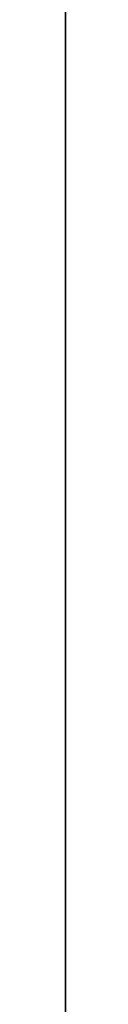
# Model space of a CAD drawing. Units: inches. Extents: x 2083 to 3317, y 1141 to 2115.
# Tile 31 of 256: x 2235.95969 to 2235.95984, y 1477.76912 to 1477.77958. Entities that reach past the tile are written whole.
import ezdxf

# ---------------------------------------------------------------- set-up
doc = ezdxf.new("R2010")
doc.units = ezdxf.units.IN
doc.layers.add('A-ANNO-DIMS', color=2, linetype='Continuous', lineweight=18)
doc.layers.add('A-WALL', color=7, linetype='Continuous', lineweight=35)
doc.layers.add('A-WALL-PATT', color=251, linetype='Continuous', lineweight=13, true_color=0x636466)
doc.styles.get("Standard").update_dxf_attribs({"font": 'arial.ttf'})
doc.dimstyles.new('ISO-25', dxfattribs={"dimtxt": 12, "dimasz": 12, "dimexe": 1.25, "dimexo": 0.625, "dimtad": 1, "dimlunit": 3, "dimtxsty": 'Standard', "dimcen": 2.5, "dimadec": 0, "dimazin": 0, "dimtfac": 1, "dimtmove": 0, "dimatfit": 3, "dimfxl": 1, "dimarcsym": 0})

# ---------------------------------------------------------------- blocks, each defined once
blk = doc.blocks.new('*D30')
at = {"layer": 'A-ANNO-DIMS', "color": 0, "lineweight": -2, "transparency": 16777216}
for p, q in [((2240.017856, 1445.273807), (2240.017856, 1448.045528)), ((2254.329327, 1445.273807), (2254.329327, 1448.045528)), ((2228.017856, 1446.795528), (2216.017856, 1446.795528)), ((2240.017856, 1446.795528), (2254.329327, 1446.795528)), ((2266.329327, 1446.795528), (2413.764866, 1446.795528))]:
    blk.add_line(p, q, dxfattribs=at)
at = {"layer": 'A-ANNO-DIMS', "color": 0, "transparency": 16777216}
for points in [[(2228.017856, 1448.795528), (2228.017856, 1444.795528), (2240.017856, 1446.795528)], [(2266.329327, 1448.795528), (2266.329327, 1444.795528), (2254.329327, 1446.795528)]]:
    blk.add_solid(points, dxfattribs=at)
at = {"layer": 'Defpoints', "color": 0, "transparency": 16777216}
for p in [(2254.329327, 1446.795528), (2240.017856, 1444.648807), (2254.329327, 1444.648807)]:
    blk.add_point(p, dxfattribs=at)
at = {"layer": 'A-ANNO-DIMS', "color": 0, "transparency": 16777216, "insert": (2346.047096, 1453.625167), "char_height": 12, "attachment_point": 5}
blk.add_mtext('WC 1\'-2 1/2" TYP.', dxfattribs=at)
blk = doc.blocks.new('*D31')
at = {"layer": 'A-ANNO-DIMS', "color": 0, "lineweight": -2, "transparency": 16777216}
for p, q in [((2237.871136, 1456.648807), (2237.871136, 1541.915179)), ((2239.392856, 1444.648807), (2236.621136, 1444.648807)), ((2237.871136, 1431.547542), (2237.871136, 1444.648807)), ((2239.392856, 1431.547542), (2236.621136, 1431.547542)), ((2237.871136, 1419.547542), (2237.871136, 1407.547542))]:
    blk.add_line(p, q, dxfattribs=at)
at = {"layer": 'A-ANNO-DIMS', "color": 0, "transparency": 16777216}
for points in [[(2235.871136, 1456.648807), (2239.871136, 1456.648807), (2237.871136, 1444.648807)], [(2235.871136, 1419.547542), (2239.871136, 1419.547542), (2237.871136, 1431.547542)]]:
    blk.add_solid(points, dxfattribs=at)
at = {"layer": 'Defpoints', "color": 0, "transparency": 16777216}
for p in [(2237.871136, 1444.648807), (2240.017856, 1444.648807), (2240.017856, 1431.547542)]:
    blk.add_point(p, dxfattribs=at)
at = {"layer": 'A-ANNO-DIMS', "color": 0, "transparency": 16777216, "insert": (2231.217486, 1505.281993), "char_height": 12, "attachment_point": 5, "rotation": 90}
blk.add_mtext('1\'-1" TYP.', dxfattribs=at)
blk = doc.blocks.new('*D45')
at = {"layer": 'A-ANNO-DIMS', "color": 0, "lineweight": -2, "transparency": 16777216}
for p, q in [((2235.959783, 1478.38636), (2235.959783, 1531.36136)), ((2418.959783, 1478.38636), (2418.959783, 1531.36136)), ((2247.959783, 1530.11136), (2406.959783, 1530.11136))]:
    blk.add_line(p, q, dxfattribs=at)
at = {"layer": 'A-ANNO-DIMS', "color": 0, "transparency": 16777216}
for points in [[(2247.959783, 1532.11136), (2247.959783, 1528.11136), (2235.959783, 1530.11136)], [(2406.959783, 1532.11136), (2406.959783, 1528.11136), (2418.959783, 1530.11136)]]:
    blk.add_solid(points, dxfattribs=at)
at = {"layer": 'Defpoints', "color": 0, "transparency": 16777216}
for p in [(2418.959783, 1530.11136), (2235.959783, 1477.76136), (2418.959783, 1477.76136)]:
    blk.add_point(p, dxfattribs=at)
at = {"layer": 'A-ANNO-DIMS', "color": 0, "transparency": 16777216, "insert": (2327.459783, 1536.867329), "char_height": 12, "attachment_point": 5}
blk.add_mtext('15\'-3"', dxfattribs=at)
blk = doc.blocks.new('*D62')
at = {"layer": 'A-ANNO-DIMS', "color": 0, "lineweight": -2, "transparency": 16777216}
for p, q in [((2235.959783, 1469.38636), (2235.959783, 1522.36136)), ((2379.959783, 1469.38636), (2379.959783, 1522.36136)), ((2247.959783, 1521.11136), (2367.959783, 1521.11136))]:
    blk.add_line(p, q, dxfattribs=at)
at = {"layer": 'A-ANNO-DIMS', "color": 0, "transparency": 16777216}
for points in [[(2247.959783, 1523.11136), (2247.959783, 1519.11136), (2235.959783, 1521.11136)], [(2367.959783, 1523.11136), (2367.959783, 1519.11136), (2379.959783, 1521.11136)]]:
    blk.add_solid(points, dxfattribs=at)
at = {"layer": 'Defpoints', "color": 0, "transparency": 16777216}
for p in [(2379.959783, 1521.11136), (2235.959783, 1468.76136), (2379.959783, 1468.76136)]:
    blk.add_point(p, dxfattribs=at)
at = {"layer": 'A-ANNO-DIMS', "color": 0, "transparency": 16777216, "insert": (2307.959783, 1527.863236), "char_height": 12, "attachment_point": 5}
blk.add_mtext('12\'-0"', dxfattribs=at)

msp = doc.modelspace()

# ---------------------------------------------------------------- hatches: boundary and pattern name
at = {"layer": 'A-WALL-PATT'}
h = msp.add_hatch(color=256, dxfattribs=at)
h.dxf.hatch_style = 1
h.paths.add_polyline_path([(3126.959783, 2020.76136), (2748.959783, 2020.76136), (2604.959783, 2020.76136), (2226.959783, 2020.76136), (2226.959783, 1702.76136), (2466.959783, 1702.76136), (2466.959783, 1582.76136), (2418.959783, 1582.76136), (2418.959783, 1477.76136), (2226.959783, 1477.76136), (2226.959783, 1263.26136), (2544.959783, 1263.26136), (2544.959783, 1411.76136), (2604.959783, 1411.76136), (2685.959783, 1411.76136), (2685.959783, 1420.76136), (2604.959783, 1420.76136), (2604.959783, 1573.76136), (2604.959783, 1702.76136), (2604.959783, 2011.76136), (2748.959783, 2011.76136), (2748.959783, 1702.76136), (2862.959783, 1702.76136), (2862.959783, 1621.76136), (2871.959783, 1621.76136), (2871.959783, 1702.76136), (2883.959783, 1702.76136), (2883.959783, 1706.939459, -0.026459), (2883.959783, 1711.76136), (2757.959783, 1711.76136), (2757.959783, 1807.76136), (2787.959783, 1807.76136), (2787.959783, 1812.26136), (2757.959783, 1812.26136), (2757.959783, 2011.76136), (2877.959783, 2011.76136), (2877.959783, 1812.26136), (2847.959783, 1812.26136), (2847.959783, 1807.76136), (2889.835742, 1807.76136), (2889.835742, 1812.26136), (2882.459783, 1812.26136), (2882.459783, 2011.76136), (3117.959783, 2011.76136), (3117.959783, 1812.26136), (2937.835742, 1812.26136), (2937.835742, 1807.76136), (2995.709783, 1807.76136), (2995.709783, 1796.117666), (3000.209783, 1796.117666), (3000.209783, 1807.76136), (3117.959783, 1807.76136), (3117.959783, 1711.76136), (3000.209783, 1711.76136), (3000.209783, 1760.117666), (2998.572705, 1760.117666, -0.020711), (2995.709783, 1760.117666), (2995.709783, 1711.76136), (2931.959783, 1711.76136), (2931.959783, 1702.76136), (3126.959783, 1702.76136)])
h.paths.add_polyline_path([(2471.459783, 2011.76136), (2471.459783, 1810.01136), (2462.716936, 1810.01136), (2462.716936, 1805.51136), (2505.959783, 1805.51136), (2505.959783, 1810.01136), (2475.959783, 1810.01136), (2475.959783, 2011.76136), (2595.959783, 2011.76136), (2595.959783, 1810.01136), (2565.959783, 1810.01136), (2565.959783, 1805.51136), (2595.959783, 1805.51136), (2595.959783, 1711.76136), (2235.959783, 1711.76136), (2235.959783, 1805.51136), (2353.709783, 1805.51136), (2353.709783, 1796.054162), (2358.209783, 1796.054162), (2358.209783, 1805.51136), (2414.716936, 1805.51136), (2414.716936, 1810.01136), (2235.959783, 1810.01136), (2235.959783, 2011.76136)], flags=16)
h.paths.add_polyline_path([(2270.204734, 1994.610008), (2270.204734, 1970.610008), (2246.204734, 1970.610008), (2246.204734, 1994.610008)], flags=0)
edge = h.paths.add_edge_path(flags=0)
edge.add_ellipse((2332.027391, 1899.798176), major_axis=(-3.042994, 3.042994), ratio=0.16825245, start_angle=-161.332166, end_angle=-156.307114, ccw=False)
edge.add_ellipse((2333.082037, 1898.74353), major_axis=(-1.054646, 1.054646), ratio=0.4535321, start_angle=-123.371019, end_angle=-94.159107)
edge = h.paths.add_edge_path(flags=0)
edge.add_ellipse((2332.027391, 1968.87629), major_axis=(3.042994, 3.042994), ratio=0.16825245, start_angle=18.667834, end_angle=23.692886)
edge.add_spline(control_points=[(2332.925596, 1970.691105), (2332.226768, 1970.3361), (2330.893709, 1969.658905), (2328.41308, 1970.932138), (2327.203934, 1967.748712), (2324.709596, 1969.955589), (2322.532822, 1967.012354), (2320.012846, 1971.295812), (2317.680308, 1968.157845), (2316.040526, 1967.102047), (2315.426904, 1966.809602)], knot_values=[0, 0, 0, 0, 2.267059, 4.324559, 6.685584, 8.878641, 11.121502, 14.300359, 17.755284, 19.732645, 19.732645, 19.732645, 19.732645], degree=3, periodic=0)
edge.add_ellipse((2332.027391, 1968.87629), major_axis=(3.042994, 3.042994), ratio=0.16825245, start_angle=18.667834, end_angle=23.692886, ccw=False)
edge.add_ellipse((2333.082037, 1969.930936), major_axis=(1.054646, 1.054646), ratio=0.4535321, start_angle=56.628981, end_angle=85.840893, ccw=False)
edge = h.paths.add_edge_path(flags=0)
edge.add_spline(control_points=[(2296.428287, 1967.987908), (2293.627804, 1965.336314), (2287.703624, 1959.727094), (2299.74386, 1949.995699), (2294.532591, 1935.668528), (2290.573228, 1920.603512), (2293.394124, 1909.973691), (2296.185407, 1904.966543)], knot_values=[0.099185, 0.099185, 0.099185, 0.099185, 0.345301, 0.619822, 0.982653, 1.386093, 1.810555, 1.810555, 1.810555, 1.810555], degree=3, periodic=0)
edge.add_spline(control_points=[(2296.185407, 1904.966543), (2297.383582, 1902.6193), (2298.000969, 1901.949312), (2298.55297, 1901.468155)], knot_values=[0.006246, 0.006246, 0.006246, 0.006246, 0.055476, 0.055476, 0.055476, 0.055476], degree=3, periodic=0)
edge.add_spline(control_points=[(2298.55297, 1901.468155), (2297.258612, 1900.923224), (2295.225294, 1900.232126), (2293.060229, 1900.614205), (2292.101423, 1900.788415), (2292.089578, 1900.790568)], knot_values=[0.312835, 0.312835, 0.312835, 0.312835, 0.40178, 0.474987, 0.475903, 0.475903, 0.475903, 0.475903], degree=3, periodic=0)
edge.add_arc((2292.793646, 1904.664109), 3.937008, 215.420897, 259.698179, ccw=False)
edge.add_spline(control_points=[(2289.585314, 1902.382304), (2289.476652, 1902.535087), (2289.36848, 1902.688035), (2289.260865, 1902.84117)], knot_values=[0.102872, 0.102872, 0.102872, 0.102872, 0.116896, 0.116896, 0.116896, 0.116896], degree=3, periodic=0)
edge.add_spline(control_points=[(2289.260865, 1902.84117), (2288.686604, 1902.550192), (2287.640048, 1902.019902), (2285.881337, 1901.873954), (2283.852972, 1901.504352), (2281.719987, 1899.710538), (2278.466991, 1899.492942), (2276.157136, 1901.883202), (2272.258953, 1899.804071), (2267.777605, 1901.843183), (2262.243882, 1900.184033), (2257.414927, 1901.782061), (2254.318374, 1900.72612), (2253.178285, 1900.337343)], knot_values=[0, 0, 0, 0, 1.907977, 3.477176, 5.261074, 7.972851, 11.680248, 13.717921, 16.939592, 22.789562, 27.502503, 33.595215, 37.145618, 37.145618, 37.145618, 37.145618], degree=3, periodic=0)
edge.add_line((2253.178285, 1900.337343), (2250.24424, 1902.84117))
edge.add_line((2250.24424, 1902.84117), (2250.24424, 1965.833296))
edge.add_line((2250.24424, 1965.833296), (2253.178285, 1968.337123))
edge.add_spline(control_points=[(2253.178285, 1968.337123), (2254.318374, 1967.948346), (2257.414927, 1966.892405), (2262.243882, 1968.490433), (2267.777605, 1966.831283), (2271.52673, 1968.537217), (2273.875914, 1967.828289), (2274.206701, 1967.727642)], knot_values=[0, 0, 0, 0, 0.09018, 0.244935, 0.364644, 0.513233, 0.537855, 0.537855, 0.537855, 0.537855], degree=3, periodic=0)
edge.add_arc((2274.352887, 1963.793349), 3.937008, 72.051134, 92.127949, ccw=False)
edge.add_arc((2281.296933, 1985.230003), 18.596298, 252.0511336, 288.5657217)
edge.add_arc((2292.316717, 1956.02888), 12.646081, 71.0267879, 113.7782184, ccw=False)
edge = h.paths.add_edge_path(flags=0)
edge.add_spline(control_points=[(2274.899415, 1951.856195), (2275.066156, 1951.616592), (2275.232687, 1951.376588), (2275.397987, 1951.135855)], knot_values=[1.409916, 1.409916, 1.409916, 1.409916, 1.43159, 1.43159, 1.43159, 1.43159], degree=3, periodic=0)
edge.add_spline(control_points=[(2275.397987, 1951.135855), (2275.792106, 1950.561885), (2276.179231, 1949.983774), (2276.545546, 1949.397103)], knot_values=[1.358238, 1.358238, 1.358238, 1.358238, 1.409916, 1.409916, 1.409916, 1.409916], degree=3, periodic=0)
edge.add_line((2276.545546, 1949.397103), (2277.437289, 1947.862185))
edge.add_spline(control_points=[(2277.437289, 1947.862185), (2276.303834, 1945.673115), (2274.639698, 1942.426882), (2274.631615, 1938.0939), (2272.799124, 1930.85155), (2274.356426, 1943.897046), (2275.947681, 1947.923356), (2276.545546, 1949.397103)], knot_values=[0.005632, 0.005632, 0.005632, 0.005632, 0.186014, 0.266002, 0.357087, 0.59639, 0.739732, 0.739732, 0.739732, 0.739732], degree=3, periodic=0)
edge.add_spline(control_points=[(2276.545546, 1949.397103), (2276.179231, 1949.983774), (2275.792106, 1950.561885), (2275.397987, 1951.135855)], knot_values=[1.358238, 1.358238, 1.358238, 1.358238, 1.409916, 1.409916, 1.409916, 1.409916], degree=3, periodic=0)
edge.add_spline(control_points=[(2275.397987, 1951.135855), (2274.9425, 1950.080452), (2274.20776, 1948.025272), (2273.934602, 1944.851477), (2272.468534, 1937.627489), (2273.466216, 1945.696466), (2274.700615, 1951.059472), (2274.899415, 1951.856195)], knot_values=[0.104364, 0.104364, 0.104364, 0.104364, 0.189636, 0.269624, 0.36071, 0.600013, 0.644622, 0.644622, 0.644622, 0.644622], degree=3, periodic=0)
h.paths.add_polyline_path([(2269.167514, 1963.127573, -0.357527), (2268.170633, 1960.97637, -0.092561), (2268.170633, 1939.436325, -0.357527), (2269.167514, 1937.285122, -0.357527), (2267.01631, 1938.282002, -0.164785), (2254.685581, 1938.282002, -0.357527), (2252.534378, 1937.285122, -0.357527), (2253.531259, 1939.436325, -0.092561), (2253.531259, 1960.97637, -0.357527), (2252.534378, 1963.127573, -0.357527), (2254.685581, 1962.130692, -0.164785), (2267.01631, 1962.130692, -0.357527)], flags=0)
h.paths.add_polyline_path([(2248.874068, 1967.8018), (2248.874068, 1957.02771), (2249.457783, 1957.02771), (2249.457783, 1911.646756), (2248.874068, 1911.646756), (2248.874068, 1900.872666), (2246.511863, 1900.872666, 0.197327), (2244.149658, 1902.456873), (2244.149658, 1966.217592, 0.197327), (2246.511863, 1967.8018)], flags=0)
h.paths.add_polyline_path([(2269.167514, 1931.389344, -0.357527), (2268.170633, 1929.238141, -0.092561), (2268.170633, 1907.698096, -0.357527), (2269.167514, 1905.546893, -0.357527), (2267.01631, 1906.543774, -0.164785), (2254.685581, 1906.543774, -0.357527), (2252.534378, 1905.546893, -0.357527), (2253.531259, 1907.698096, -0.092561), (2253.531259, 1929.238141, -0.357527), (2252.534378, 1931.389344, -0.357527), (2254.685581, 1930.392463, -0.164785), (2267.01631, 1930.392463, -0.357527)], flags=0)
edge = h.paths.add_edge_path(flags=0)
edge.add_spline(control_points=[(2276.196858, 1906.723702), (2276.168144, 1909.028928), (2276.114049, 1913.371852), (2270.598417, 1924.924978), (2273.905175, 1919.012779), (2275.921711, 1916.262063), (2275.47457, 1912.402149), (2277.257874, 1910.380621), (2276.696044, 1908.225036), (2276.646218, 1906.813023), (2276.617825, 1906.008407)], knot_values=[0, 0, 0, 0, 8.61026, 16.221274, 18.843057, 23.804898, 27.440828, 29.356102, 31.203478, 33.650687, 33.650687, 33.650687, 33.650687], degree=3, periodic=0)
edge.add_spline(control_points=[(2276.617825, 1906.008407), (2276.623313, 1905.624144), (2276.497738, 1904.628661), (2275.441779, 1903.854725), (2274.937314, 1903.08045), (2274.85908, 1902.84117)], knot_values=[0.156488, 0.156488, 0.156488, 0.156488, 0.184398, 0.231376, 0.250598, 0.250598, 0.250598, 0.250598], degree=3, periodic=0)
edge.add_line((2274.85908, 1902.84117), (2276.50598, 1902.84117))
edge.add_spline(control_points=[(2276.50598, 1902.84117), (2276.788308, 1903.08494), (2277.665071, 1904.125196), (2278.249538, 1904.340738), (2277.653872, 1908.527387), (2278.15567, 1906.227808), (2278.100464, 1905.285948), (2278.846675, 1904.069005), (2277.856785, 1903.414948), (2277.874191, 1902.99105), (2277.903562, 1902.84117)], knot_values=[0.059574, 0.059574, 0.059574, 0.059574, 0.080753, 0.103741, 0.16972, 0.176036, 0.207137, 0.240474, 0.262341, 0.27366, 0.27366, 0.27366, 0.27366], degree=3, periodic=0)
edge.add_line((2277.903562, 1902.84117), (2280.029825, 1902.84117))
edge.add_spline(control_points=[(2280.029825, 1902.84117), (2279.888221, 1903.088398), (2279.499257, 1903.981551), (2280.152284, 1905.939349), (2278.103615, 1909.657757), (2279.762395, 1907.185285), (2280.3279, 1904.874861), (2280.485109, 1903.48959), (2281.463269, 1903.249432), (2281.758343, 1902.936497), (2281.834036, 1902.84117)], knot_values=[0.013856, 0.013856, 0.013856, 0.013856, 0.034874, 0.088867, 0.107879, 0.126738, 0.158714, 0.193757, 0.217487, 0.226722, 0.226722, 0.226722, 0.226722], degree=3, periodic=0)
edge.add_spline(control_points=[(2281.834036, 1902.84117), (2281.787535, 1902.826703), (2281.647022, 1902.782988), (2281.395527, 1902.85949), (2281.088077, 1902.985242), (2280.720683, 1903.060902), (2280.333451, 1903.025726), (2280.124767, 1902.898879), (2280.029825, 1902.84117)], knot_values=[0, 0, 0, 0, 0.14413, 0.435517, 0.749276, 1.153046, 1.548371, 1.878348, 1.878348, 1.878348, 1.878348], degree=3, periodic=0)
edge.add_line((2280.029825, 1902.84117), (2277.903562, 1902.84117))
edge.add_spline(control_points=[(2277.903562, 1902.84117), (2277.892855, 1902.795855), (2277.865396, 1902.679637), (2277.607479, 1902.687483), (2277.27405, 1902.8007), (2276.837921, 1902.619775), (2276.583807, 1902.789261), (2276.50598, 1902.84117)], knot_values=[0, 0, 0, 0, 0.127189, 0.326199, 0.628009, 1.24357, 1.515331, 1.515331, 1.515331, 1.515331], degree=3, periodic=0)
edge.add_line((2276.50598, 1902.84117), (2274.85908, 1902.84117))
edge.add_spline(control_points=[(2274.85908, 1902.84117), (2274.814437, 1902.898587), (2274.72513, 1903.013446), (2274.493477, 1903.118968), (2274.244285, 1902.960539), (2273.937121, 1903.184942), (2273.614039, 1902.983143), (2273.408316, 1902.883045), (2273.322254, 1902.84117)], knot_values=[0, 0, 0, 0, 0.21843, 0.436957, 0.687977, 0.990379, 1.398396, 1.69185, 1.69185, 1.69185, 1.69185], degree=3, periodic=0)
edge.add_spline(control_points=[(2273.322254, 1902.84117), (2273.61674, 1903.445692), (2274.273998, 1904.538253), (2276.027239, 1904.573702), (2276.206963, 1906.583637), (2276.196858, 1906.723702)], knot_values=[0.012227, 0.012227, 0.012227, 0.012227, 0.059472, 0.106218, 0.134458, 0.134458, 0.134458, 0.134458], degree=3, periodic=0)
h.paths.add_polyline_path([(2270.776054, 1897.789828), (2270.776054, 1873.789828), (2246.776054, 1873.789828), (2246.776054, 1897.789828)], flags=0)
h.paths.add_polyline_path([(2353.709783, 1760.005059), (2353.709783, 1760.054162), (2358.209783, 1760.054162, -0.033729)], flags=0)
h.paths.add_polyline_path([(2321.819119, 1737.529186), (2341.995327, 1737.529186, -0.414214), (2343.203273, 1736.321241), (2343.203273, 1721.020596, -0.414214), (2341.995327, 1719.812651), (2321.819119, 1719.812651, -0.414214), (2320.611173, 1721.020596), (2320.611173, 1736.321241, -0.414214)], flags=0)
h.paths.add_polyline_path([(2324.23501, 1736.321241), (2339.579436, 1736.321241, -0.414214), (2341.995327, 1733.905349), (2341.995327, 1725.44973, -0.414214), (2339.579436, 1723.033839), (2333.680588, 1723.033839), (2333.845317, 1722.045467, -0.870646), (2335.425399, 1721.825893, -0.767327), (2333.922694, 1721.423245), (2331.291024, 1721.423245, -0.767327), (2329.788319, 1721.825893, -0.870646), (2331.368401, 1722.045467), (2331.53313, 1723.033839), (2324.23501, 1723.033839, -0.414214), (2321.819119, 1725.44973), (2321.819119, 1733.905349, -0.414214)], flags=0)
h.paths.add_polyline_path([(2570.483789, 1928.615444), (2589.683789, 1928.615444), (2590.168829, 1928.615444), (2590.168829, 1904.993397), (2570.483789, 1904.993397)], flags=0)
h.paths.add_polyline_path([(2574.447324, 1927.263822, -1), (2572.828836, 1927.263822, -1)], flags=0)
h.paths.add_polyline_path([(2573.089867, 1926.940877), (2573.925032, 1927.776042), (2574.147743, 1927.553332), (2573.312577, 1926.718166)], flags=0)
h.paths.add_polyline_path([(2578.779065, 1919.729618, -1), (2571.591663, 1919.729618, -1)], flags=0)
h.paths.add_polyline_path([(2578.385364, 1919.729618, -1), (2571.985364, 1919.729618, -1)], flags=0)
h.paths.add_polyline_path([(2331.595764, 1729.476216, -1), (2333.617954, 1729.476216, -1)], flags=0)
h.paths.add_polyline_path([(2578.034228, 1927.263822, -1), (2576.41574, 1927.263822, -1)], flags=0)
h.paths.add_polyline_path([(2576.688851, 1927.531089), (2576.911562, 1927.753799), (2577.746728, 1926.918634), (2577.524017, 1926.695923)], flags=0)
h.paths.add_polyline_path([(2578.139065, 1909.859539, -1), (2572.231663, 1909.859539, -1)], flags=0)
h.paths.add_polyline_path([(2577.745364, 1909.859539, -1), (2572.625364, 1909.859539, -1)], flags=0)
h.paths.add_polyline_path([(2583.797718, 1927.263822, -1), (2582.179229, 1927.263822, -1)], flags=0)
h.paths.add_polyline_path([(2582.718649, 1927.753799), (2583.553814, 1926.918634), (2583.331103, 1926.695923), (2582.495938, 1927.531089)], flags=0)
h.paths.add_polyline_path([(2582.495938, 1927.531089), (2582.718649, 1927.753799), (2583.553814, 1926.918634), (2583.331103, 1926.695923)], flags=0)
h.paths.add_polyline_path([(2587.739065, 1920.529618, -1), (2581.831663, 1920.529618, -1)], flags=0)
h.paths.add_polyline_path([(2587.345364, 1920.529618, -1), (2582.225364, 1920.529618, -1)], flags=0)
h.paths.add_polyline_path([(2587.384622, 1927.263822, -1), (2585.766133, 1927.263822, -1)], flags=0)
h.paths.add_polyline_path([(2586.081993, 1926.980247), (2586.917158, 1927.815412), (2587.139869, 1927.592702), (2586.304703, 1926.757536)], flags=0)
h.paths.add_polyline_path([(2588.379065, 1910.659539, -1), (2581.191663, 1910.659539, -1)], flags=0)
h.paths.add_polyline_path([(2587.985364, 1910.659539, -1), (2581.585364, 1910.659539, -1)], flags=0)
h.paths.add_polyline_path([(2417.167729, 1729.477895), (2437.343937, 1729.477895, -0.414214), (2438.551883, 1728.26995), (2438.551883, 1712.969306, -0.414214), (2437.343937, 1711.76136), (2417.167729, 1711.76136, -0.414214), (2415.959783, 1712.969306), (2415.959783, 1728.26995, -0.414214)], flags=0)
h.paths.add_polyline_path([(2419.58362, 1728.26995), (2434.928046, 1728.26995, -0.414214), (2437.343937, 1725.854059), (2437.343937, 1717.39844, -0.414214), (2434.928046, 1714.982548), (2429.029199, 1714.982548), (2429.193927, 1713.994176, -0.870646), (2430.774009, 1713.774603, -0.767327), (2429.271304, 1713.371954), (2426.639634, 1713.371954, -0.767327), (2425.136929, 1713.774603, -0.870646), (2426.717011, 1713.994176), (2426.88174, 1714.982548), (2419.58362, 1714.982548, -0.414214), (2417.167729, 1717.39844), (2417.167729, 1725.854059, -0.414214)], flags=0)
h.paths.add_polyline_path([(2419.58362, 1728.26995), (2434.928046, 1728.26995, -0.414214), (2437.343937, 1725.854059), (2437.343937, 1717.39844, -0.414214), (2434.928046, 1714.982548), (2429.029199, 1714.982548), (2428.358118, 1719.009034), (2427.552821, 1719.009034), (2426.88174, 1714.982548), (2419.58362, 1714.982548, -0.414214), (2417.167729, 1717.39844), (2417.167729, 1725.854059, -0.414214)], flags=0)
h.paths.add_polyline_path([(2426.944374, 1721.424925, -1), (2428.966564, 1721.424925, -1)], flags=0)
h.paths.add_polyline_path([(2475.959783, 1702.76136), (2595.959783, 1702.76136), (2595.959783, 1582.76136), (2475.959783, 1582.76136)], flags=16)
h.paths.add_polyline_path([(2427.959783, 1573.76136), (2595.959783, 1573.76136), (2595.959783, 1468.76136), (2595.959783, 1420.76136), (2384.459783, 1420.76136), (2384.459783, 1468.76136), (2427.959783, 1468.76136)], flags=16)
h.paths.add_polyline_path([(2379.959783, 1468.76136), (2379.959783, 1420.76136), (2235.959783, 1420.76136), (2235.959783, 1468.76136)], flags=16)
h.paths.add_polyline_path([(2317.815996, 1466.695767), (2337.992205, 1466.695767, -0.414214), (2339.20015, 1465.487821), (2339.20015, 1450.187177, -0.414214), (2337.992205, 1448.979232), (2317.815996, 1448.979232, -0.414214), (2316.608051, 1450.187177), (2316.608051, 1465.487821, -0.414214)], flags=0)
h.paths.add_polyline_path([(2320.231887, 1465.487821), (2335.576313, 1465.487821, -0.414214), (2337.992205, 1463.07193), (2337.992205, 1454.616311, -0.414214), (2335.576313, 1452.20042), (2329.677466, 1452.20042), (2329.842195, 1451.212047, -0.870646), (2331.422276, 1450.992474, -0.767327), (2329.919571, 1450.589826), (2327.287902, 1450.589826, -0.767327), (2325.785197, 1450.992474, -0.870646), (2327.365278, 1451.212047), (2327.530007, 1452.20042), (2320.231887, 1452.20042, -0.414214), (2317.815996, 1454.616311), (2317.815996, 1463.07193, -0.414214)], flags=0)
h.paths.add_polyline_path([(2320.231887, 1465.487821), (2335.576313, 1465.487821, -0.414214), (2337.992205, 1463.07193), (2337.992205, 1454.616311, -0.414214), (2335.576313, 1452.20042), (2329.677466, 1452.20042), (2329.006385, 1456.226905), (2328.201088, 1456.226905), (2327.530007, 1452.20042), (2320.231887, 1452.20042, -0.414214), (2317.815996, 1454.616311), (2317.815996, 1463.07193, -0.414214)], flags=0)
h.paths.add_polyline_path([(2327.592641, 1458.642796, -1), (2329.614832, 1458.642796, -1)], flags=0)
h.paths.add_polyline_path([(2244.411744, 1433.340453), (2241.920945, 1433.340453, -0.414214), (2240.017856, 1435.243542), (2240.017856, 1440.952808, -0.414211), (2241.920925, 1442.855897), (2244.411744, 1442.855897, -1.976472)], flags=0)
h.paths.add_polyline_path([(2245.356888, 1434.397536, -0.414214), (2245.356888, 1441.798814, -2.144098)], flags=0)
h.paths.add_polyline_path([(2535.959783, 1416.26136), (2535.959783, 1272.26136), (2235.959783, 1272.26136), (2235.959783, 1416.26136)], flags=16)
h.paths.add_polyline_path([(2260.119561, 1384.292841), (2260.119561, 1362.038649), (2237.865369, 1362.038649), (2237.865369, 1384.292841)], flags=0)
edge = h.paths.add_edge_path(flags=0)
edge.add_line((2318.251847, 1362.093298), (2318.145797, 1362.000973))
edge.add_ellipse((2317.445116, 1360.431044), major_axis=(2.82164, 2.82164), ratio=0.16825245, start_angle=18.667834, end_angle=20.948127, ccw=False)
edge.add_ellipse((2318.423045, 1361.408974), major_axis=(0.977929, 0.977929), ratio=0.4535321, start_angle=56.628981, end_angle=70.226201, ccw=False)
edge = h.paths.add_edge_path(flags=0)
edge.add_line((2319.10737, 1295.571078), (2319.015044, 1295.677128))
edge.add_ellipse((2317.445116, 1296.377809), major_axis=(-2.82164, 2.82164), ratio=0.16825245, start_angle=-161.332166, end_angle=-159.051873, ccw=False)
edge.add_ellipse((2318.423045, 1295.39988), major_axis=(-0.977929, 0.977929), ratio=0.4535321, start_angle=-123.371019, end_angle=-109.773799)
edge = h.paths.add_edge_path(flags=0)
edge.add_spline(control_points=[(2284.210349, 1301.170219), (2284.580688, 1300.444719), (2284.891189, 1299.892024), (2285.159553, 1299.461018)], knot_values=[0.039066, 0.039066, 0.039066, 0.039066, 0.055476, 0.055476, 0.055476, 0.055476], degree=3, periodic=0)
edge.add_line((2285.159553, 1299.461018), (2284.210349, 1301.170219))
edge = h.paths.add_edge_path(flags=0)
edge.add_line((2280.412458, 1297.298013), (2283.369991, 1297.036122))
edge.add_line((2283.369991, 1297.036122), (2286.40569, 1297.92631))
edge.add_spline(control_points=[(2286.40569, 1297.92631), (2285.305487, 1297.463119), (2284.344777, 1297.129151), (2283.369991, 1297.036122)], knot_values=[0.394369, 0.394369, 0.394369, 0.394369, 0.475903, 0.475903, 0.475903, 0.475903], degree=3, periodic=0)
edge.add_spline(control_points=[(2283.369991, 1297.036122), (2283.28139, 1297.027666), (2282.316289, 1296.957336), (2281.312502, 1297.134479), (2280.423441, 1297.296016), (2280.412458, 1297.298013)], knot_values=[0.312835, 0.312835, 0.312835, 0.312835, 0.320246, 0.393453, 0.394369, 0.394369, 0.394369, 0.394369], degree=3, periodic=0)
edge = h.paths.add_edge_path(flags=0)
edge.add_line((2284.435561, 1359.607285), (2280.446291, 1355.328047))
edge.add_line((2280.446291, 1355.328047), (2279.579987, 1351.017754))
edge.add_line((2279.579987, 1351.017754), (2282.412974, 1346.580433))
edge.add_spline(control_points=[(2282.412974, 1346.580433), (2283.153331, 1345.589236), (2284.252896, 1344.028897), (2284.801037, 1342.387167), (2284.935162, 1341.805544)], knot_values=[1.240098, 1.240098, 1.240098, 1.240098, 1.332892, 1.382712, 1.382712, 1.382712, 1.382712], degree=3, periodic=0)
edge.add_spline(control_points=[(2284.935162, 1341.805544), (2285.319108, 1340.1406), (2285.233029, 1338.409204), (2284.909938, 1336.654122)], knot_values=[1.097484, 1.097484, 1.097484, 1.097484, 1.240098, 1.240098, 1.240098, 1.240098], degree=3, periodic=0)
edge.add_spline(control_points=[(2284.909938, 1336.654122), (2284.586848, 1334.89904), (2284.026745, 1333.120272), (2283.462644, 1331.360585)], knot_values=[0.95487, 0.95487, 0.95487, 0.95487, 1.097484, 1.097484, 1.097484, 1.097484], degree=3, periodic=0)
edge.add_line((2283.462644, 1331.360585), (2281.890376, 1326.153357))
edge.add_line((2281.890376, 1326.153357), (2280.756259, 1321.056089))
edge.add_line((2280.756259, 1321.056089), (2280.299205, 1316.001977))
edge.add_line((2280.299205, 1316.001977), (2280.715933, 1310.950068))
edge.add_line((2280.715933, 1310.950068), (2282.028094, 1305.972137))
edge.add_line((2282.028094, 1305.972137), (2284.210349, 1301.170219))
edge.add_spline(control_points=[(2284.210349, 1301.170219), (2283.340731, 1302.730185), (2282.611904, 1304.336493), (2282.028094, 1305.972137)], knot_values=[0.099185, 0.099185, 0.099185, 0.099185, 0.241799, 0.241799, 0.241799, 0.241799], degree=3, periodic=0)
edge.add_spline(control_points=[(2282.028094, 1305.972137), (2281.444283, 1307.60778), (2281.005489, 1309.272759), (2280.715933, 1310.950068)], knot_values=[0.241799, 0.241799, 0.241799, 0.241799, 0.384413, 0.384413, 0.384413, 0.384413], degree=3, periodic=0)
edge.add_spline(control_points=[(2280.715933, 1310.950068), (2280.433241, 1312.587613), (2280.289386, 1314.276959), (2280.298894, 1315.962032), (2280.299205, 1316.001977)], knot_values=[0.384413, 0.384413, 0.384413, 0.384413, 0.523647, 0.527028, 0.527028, 0.527028, 0.527028], degree=3, periodic=0)
edge.add_spline(control_points=[(2280.299205, 1316.001977), (2280.312326, 1317.686955), (2280.477871, 1319.367926), (2280.756259, 1321.056089)], knot_values=[0.527028, 0.527028, 0.527028, 0.527028, 0.669642, 0.669642, 0.669642, 0.669642], degree=3, periodic=0)
edge.add_spline(control_points=[(2280.756259, 1321.056089), (2281.034648, 1322.744252), (2281.42588, 1324.439608), (2281.890376, 1326.153357)], knot_values=[0.669642, 0.669642, 0.669642, 0.669642, 0.812256, 0.812256, 0.812256, 0.812256], degree=3, periodic=0)
edge.add_spline(control_points=[(2281.890376, 1326.153357), (2282.264383, 1327.533251), (2282.78787, 1329.26181), (2283.352751, 1331.01778), (2283.462644, 1331.360585)], knot_values=[0.812256, 0.812256, 0.812256, 0.812256, 0.927087, 0.95487, 0.95487, 0.95487, 0.95487], degree=3, periodic=0)
edge.add_line((2283.462644, 1331.360585), (2284.909938, 1336.654122))
edge.add_line((2284.909938, 1336.654122), (2284.935162, 1341.805544))
edge.add_line((2284.935162, 1341.805544), (2282.412974, 1346.580433))
edge.add_spline(control_points=[(2282.412974, 1346.580433), (2281.275127, 1348.103792), (2280.078447, 1349.570318), (2279.579987, 1351.017754)], knot_values=[1.382712, 1.382712, 1.382712, 1.382712, 1.525326, 1.525326, 1.525326, 1.525326], degree=3, periodic=0)
edge.add_spline(control_points=[(2279.579987, 1351.017754), (2279.443282, 1351.414721), (2279.136312, 1352.856922), (2279.73519, 1354.290385), (2280.446291, 1355.328047)], knot_values=[1.525326, 1.525326, 1.525326, 1.525326, 1.564439, 1.667941, 1.667941, 1.667941, 1.667941], degree=3, periodic=0)
edge.add_spline(control_points=[(2280.446291, 1355.328047), (2281.426113, 1356.757835), (2282.930837, 1358.18256), (2284.435561, 1359.607285)], knot_values=[1.667941, 1.667941, 1.667941, 1.667941, 1.810555, 1.810555, 1.810555, 1.810555], degree=3, periodic=0)
edge.add_arc((2280.623075, 1348.518181), 11.72618, 71.0267879, 113.7782184)
edge.add_arc((2270.404892, 1375.595156), 17.243567, 252.0511336, 288.5657217, ccw=False)
edge.add_arc((2263.965969, 1355.717847), 3.650622, 72.051134, 92.127949)
edge.add_arc((2263.965969, 1355.717847), 3.650622, 92.127949, 177.98513)
edge.add_spline(control_points=[(2260.317604, 1355.846199), (2260.260417, 1354.220668), (2260.551278, 1350.186547), (2262.999344, 1346.766251), (2264.472741, 1344.649024)], knot_values=[1.43159, 1.43159, 1.43159, 1.43159, 1.564144, 1.770695, 1.770695, 1.770695, 1.770695], degree=3, periodic=0)
edge.add_line((2264.472741, 1344.649024), (2264.93559, 1343.98253))
edge.add_spline(control_points=[(2263.801044, 1340.248105), (2263.843238, 1340.514088), (2264.067244, 1341.756465), (2264.512693, 1343.002453), (2264.935047, 1343.981083)], knot_values=[0.53657, 0.53657, 0.53657, 0.53657, 0.559349, 0.644622, 0.644622, 0.644622, 0.644622], degree=3, periodic=0)
edge.add_spline(control_points=[(2264.935047, 1343.981083), (2265.117771, 1343.714975), (2265.298875, 1343.447906), (2265.476756, 1343.179365)], knot_values=[1.384077, 1.384077, 1.384077, 1.384077, 1.409916, 1.409916, 1.409916, 1.409916], degree=3, periodic=0)
edge.add_spline(control_points=[(2265.476756, 1343.179365), (2265.654637, 1342.910823), (2265.829296, 1342.64081), (2265.99913, 1342.368812)], knot_values=[1.358238, 1.358238, 1.358238, 1.358238, 1.384077, 1.384077, 1.384077, 1.384077], degree=3, periodic=0)
edge.add_line((2265.99913, 1342.368812), (2266.826006, 1340.945547))
edge.add_spline(control_points=[(2266.826006, 1340.945547), (2268.894401, 1337.089691), (2271.398173, 1325.843001), (2270.516164, 1310.568557), (2275.919376, 1301.860609), (2277.789511, 1299.19945)], knot_values=[0.116896, 0.116896, 0.116896, 0.116896, 0.472987, 1.050969, 1.313793, 1.313793, 1.313793, 1.313793], degree=3, periodic=0)
edge.add_spline(control_points=[(2277.789511, 1299.19945), (2277.839405, 1299.128452), (2277.889428, 1299.057498), (2277.939572, 1298.986584)], knot_values=[0.109884, 0.109884, 0.109884, 0.109884, 0.116896, 0.116896, 0.116896, 0.116896], degree=3, periodic=0)
edge.add_line((2277.939572, 1298.986584), (2277.788849, 1299.199114))
edge.add_spline(control_points=[(2277.788849, 1299.199114), (2277.256582, 1298.929414), (2276.28635, 1298.437902), (2275.039352, 1298.334419), (2274.38333, 1298.238895), (2274.215254, 1298.209338)], knot_values=[33.12187, 33.12187, 33.12187, 33.12187, 35.029056, 36.598255, 37.144827, 37.144827, 37.144827, 37.144827], degree=3, periodic=0)
edge.add_line((2274.215254, 1298.209338), (2273.073147, 1297.892961))
edge.add_spline(control_points=[(2273.073147, 1297.892961), (2272.322936, 1297.579784), (2271.039151, 1296.510508), (2269.248395, 1296.226062), (2268.4231, 1296.374654)], knot_values=[26.532584, 26.532584, 26.532584, 26.532584, 29.198919, 31.839101, 31.839101, 31.839101, 31.839101], degree=3, periodic=0)
edge.add_line((2268.4231, 1296.374654), (2263.878501, 1297.457534))
edge.add_spline(control_points=[(2263.878501, 1297.457534), (2263.556077, 1297.359435), (2261.860306, 1296.838694), (2260.23878, 1297.282407), (2258.933454, 1297.516461)], knot_values=[15.919551, 15.919551, 15.919551, 15.919551, 16.939592, 21.226067, 21.226067, 21.226067, 21.226067], degree=3, periodic=0)
edge.add_line((2258.933454, 1297.516461), (2254.055233, 1297.32901))
edge.add_spline(control_points=[(2254.055233, 1297.32901), (2253.755525, 1297.295815), (2252.113683, 1297.165174), (2250.461869, 1297.544221), (2249.129686, 1297.667882)], knot_values=[5.306517, 5.306517, 5.306517, 5.306517, 6.276435, 10.613034, 10.613034, 10.613034, 10.613034], degree=3, periodic=0)
edge.add_line((2249.129686, 1297.667882), (2244.33165, 1296.877756))
edge.add_line((2244.33165, 1296.877756), (2241.611033, 1299.19945))
edge.add_line((2241.611033, 1299.19945), (2241.611033, 1357.609404))
edge.add_line((2241.611033, 1357.609404), (2244.33165, 1359.931097))
edge.add_line((2244.33165, 1359.931097), (2252.728823, 1359.542692))
edge.add_spline(control_points=[(2252.728823, 1359.542692), (2252.870939, 1359.54644), (2253.30574, 1359.548172), (2253.739845, 1359.514274), (2254.031742, 1359.482426)], knot_values=[0.233291, 0.233291, 0.233291, 0.233291, 0.244935, 0.268927, 0.268927, 0.268927, 0.268927], degree=3, periodic=0)
edge.add_line((2254.031742, 1359.482426), (2259.58719, 1359.41639))
edge.add_spline(control_points=[(2259.58719, 1359.41639), (2260.677068, 1359.628503), (2262.073197, 1359.897003), (2263.523692, 1359.459278), (2263.830417, 1359.365952)], knot_values=[0.422516, 0.422516, 0.422516, 0.422516, 0.513233, 0.537855, 0.537855, 0.537855, 0.537855], degree=3, periodic=0)
edge.add_arc((2263.965969, 1355.717847), 3.650622, 72.051134, 92.127949, ccw=False)
edge.add_arc((2270.404892, 1375.595156), 17.243567, 252.0511336, 288.5657217)
edge.add_arc((2280.623075, 1348.518181), 11.72618, 71.0267879, 113.7782184, ccw=False)
h.paths.add_polyline_path([(2240.34053, 1359.434715), (2240.34053, 1349.444353), (2240.881785, 1349.444353), (2240.881785, 1307.3645), (2240.34053, 1307.3645), (2240.34053, 1297.374138), (2238.150157, 1297.374138, 0.197327), (2235.959783, 1298.843108), (2235.959783, 1357.965746, 0.197327), (2238.150157, 1359.434715)], flags=0)
h.paths.add_polyline_path([(2259.15779, 1355.1005, -0.357527), (2258.233425, 1353.10578, -0.092561), (2258.233425, 1333.132601, -0.357527), (2259.15779, 1331.13788, -0.357527), (2257.16307, 1332.062246, -0.164785), (2245.729302, 1332.062246, -0.357527), (2243.734582, 1331.13788, -0.357527), (2244.658947, 1333.132601, -0.092561), (2244.658947, 1353.10578, -0.357527), (2243.734582, 1355.1005, -0.357527), (2245.729302, 1354.176135, -0.164785), (2257.16307, 1354.176135, -0.357527)], flags=0)
edge = h.paths.add_edge_path(flags=0)
edge.add_line((2265.99913, 1342.368812), (2266.826006, 1340.945547))
edge.add_line((2266.826006, 1340.945547), (2265.307557, 1337.814066))
edge.add_line((2265.307557, 1337.814066), (2264.358232, 1334.652939))
edge.add_line((2264.358232, 1334.652939), (2264.262012, 1333.799705))
edge.add_spline(control_points=[(2264.262012, 1333.799705), (2264.208357, 1333.187055), (2264.16206, 1332.365525), (2264.007144, 1331.413933), (2263.969049, 1331.201834)], knot_values=[0.464444, 0.464444, 0.464444, 0.464444, 0.516691, 0.531608, 0.531608, 0.531608, 0.531608], degree=3, periodic=0)
edge.add_spline(control_points=[(2263.969049, 1331.201834), (2263.774535, 1330.118873), (2263.42437, 1328.790839), (2263.25742, 1328.530652), (2263.234028, 1328.514612)], knot_values=[0.372682, 0.372682, 0.372682, 0.372682, 0.44885, 0.464444, 0.464444, 0.464444, 0.464444], degree=3, periodic=0)
edge.add_spline(control_points=[(2263.234028, 1328.514612), (2263.096382, 1328.420227), (2263.13117, 1329.301477), (2263.274953, 1330.615749)], knot_values=[0.280919, 0.280919, 0.280919, 0.280919, 0.372682, 0.372682, 0.372682, 0.372682], degree=3, periodic=0)
edge.add_spline(control_points=[(2263.274953, 1330.615749), (2263.418736, 1331.930022), (2263.671515, 1333.677318), (2263.969852, 1335.315027)], knot_values=[0.189157, 0.189157, 0.189157, 0.189157, 0.280919, 0.280919, 0.280919, 0.280919], degree=3, periodic=0)
edge.add_spline(control_points=[(2263.969852, 1335.315027), (2264.100496, 1336.032192), (2264.418783, 1337.621911), (2264.754848, 1338.86443), (2264.947419, 1339.491124)], knot_values=[0.097394, 0.097394, 0.097394, 0.097394, 0.137578, 0.189157, 0.189157, 0.189157, 0.189157], degree=3, periodic=0)
edge.add_spline(control_points=[(2264.947419, 1339.491124), (2265.290017, 1340.606055), (2265.644238, 1341.493996), (2265.99913, 1342.368812)], knot_values=[0.005632, 0.005632, 0.005632, 0.005632, 0.097394, 0.097394, 0.097394, 0.097394], degree=3, periodic=0)
h.paths.add_polyline_path([(2259.15779, 1325.670973, -0.357527), (2258.233425, 1323.676253, -0.092561), (2258.233425, 1303.703073, -0.357527), (2259.15779, 1301.708353, -0.357527), (2257.16307, 1302.632719, -0.164785), (2245.729302, 1302.632719, -0.357527), (2243.734582, 1301.708353, -0.357527), (2244.658947, 1303.703073, -0.092561), (2244.658947, 1323.676253, -0.357527), (2243.734582, 1325.670973, -0.357527), (2245.729302, 1324.746608, -0.164785), (2257.16307, 1324.746608, -0.357527)], flags=0)
edge = h.paths.add_edge_path(flags=0)
edge.add_spline(control_points=[(2261.708938, 1317.311421), (2261.679482, 1317.41758), (2261.761858, 1317.388535), (2262.490736, 1316.089873), (2262.962185, 1315.300897)], knot_values=[14.955861, 14.955861, 14.955861, 14.955861, 16.221274, 18.694826, 18.694826, 18.694826, 18.694826], degree=3, periodic=0)
edge.add_spline(control_points=[(2262.962185, 1315.300897), (2262.990437, 1315.253617), (2263.702096, 1314.067376), (2264.348983, 1313.127153), (2264.730054, 1312.164154)], knot_values=[18.694826, 18.694826, 18.694826, 18.694826, 18.843057, 22.433791, 22.433791, 22.433791, 22.433791], degree=3, periodic=0)
edge.add_spline(control_points=[(2264.730054, 1312.164154), (2264.875565, 1311.796437), (2265.176873, 1310.769807), (2265.143069, 1309.559262), (2265.247736, 1308.824193)], knot_values=[22.433791, 22.433791, 22.433791, 22.433791, 23.804898, 26.172756, 26.172756, 26.172756, 26.172756], degree=3, periodic=0)
edge.add_line((2265.247736, 1308.824193), (2265.850774, 1307.171888))
edge.add_spline(control_points=[(2265.850774, 1307.171888), (2266.065025, 1306.821678), (2266.384387, 1306.332246), (2266.4244, 1305.780549), (2266.420369, 1305.611216)], knot_values=[28.062562, 28.062562, 28.062562, 28.062562, 29.356102, 29.911721, 29.911721, 29.911721, 29.911721], degree=3, periodic=0)
edge.add_spline(control_points=[(2266.420369, 1305.611216), (2266.416116, 1305.43259), (2266.393999, 1305.249998), (2266.364777, 1305.065857)], knot_values=[29.911721, 29.911721, 29.911721, 29.911721, 30.497837, 30.497837, 30.497837, 30.497837], degree=3, periodic=0)
edge.add_line((2266.364777, 1305.065857), (2266.066151, 1302.136295))
edge.add_spline(control_points=[(2266.066151, 1302.136295), (2266.07124, 1301.779984), (2265.998076, 1301.199985), (2265.663266, 1300.758961), (2265.508908, 1300.585882)], knot_values=[0.156488, 0.156488, 0.156488, 0.156488, 0.184398, 0.203543, 0.203543, 0.203543, 0.203543], degree=3, periodic=0)
edge.add_line((2265.508908, 1300.585882), (2264.435341, 1299.19945))
edge.add_line((2264.435341, 1299.19945), (2265.962442, 1299.19945))
edge.add_line((2265.962442, 1299.19945), (2267.33599, 1301.175276))
edge.add_line((2267.33599, 1301.175276), (2267.311667, 1301.986237))
edge.add_spline(control_points=[(2267.311667, 1301.986237), (2267.261111, 1302.862396), (2267.160212, 1303.737132), (2267.271486, 1303.325896)], knot_values=[0.126229, 0.126229, 0.126229, 0.126229, 0.166617, 0.166617, 0.166617, 0.166617], degree=3, periodic=0)
edge.add_spline(control_points=[(2267.271486, 1303.325896), (2267.280035, 1303.294305), (2267.309785, 1303.175366), (2267.37345, 1302.883608), (2267.406123, 1302.682829), (2267.417926, 1302.601025)], knot_values=[0.166617, 0.166617, 0.166617, 0.166617, 0.16972, 0.176036, 0.180765, 0.180765, 0.180765, 0.180765], degree=3, periodic=0)
edge.add_spline(control_points=[(2267.743891, 1300.987505), (2267.687583, 1301.150943), (2267.48052, 1301.656664), (2267.483751, 1302.144788), (2267.417926, 1302.601025)], knot_values=[0.180765, 0.180765, 0.180765, 0.180765, 0.193767, 0.220139, 0.220139, 0.220139, 0.220139], degree=3, periodic=0)
edge.add_line((2267.417926, 1302.601025), (2267.743891, 1300.987505))
edge.add_spline(control_points=[(2267.743891, 1300.987505), (2267.831961, 1300.731878), (2267.932021, 1300.309904), (2267.554841, 1299.974518), (2267.429366, 1299.829207)], knot_values=[0.220139, 0.220139, 0.220139, 0.220139, 0.240474, 0.25489, 0.25489, 0.25489, 0.25489], degree=3, periodic=0)
edge.add_line((2267.429366, 1299.829207), (2267.258361, 1299.19945))
edge.add_line((2267.258361, 1299.19945), (2269.229956, 1299.19945))
edge.add_spline(control_points=[(2269.229956, 1299.19945), (2269.098653, 1299.428694), (2268.842774, 1300.016251), (2269.011575, 1300.915923), (2268.946796, 1301.66074)], knot_values=[0.013856, 0.013856, 0.013856, 0.013856, 0.034874, 0.067073, 0.067073, 0.067073, 0.067073], degree=3, periodic=0)
edge.add_line((2268.946796, 1301.66074), (2268.431582, 1303.603109))
edge.add_spline(control_points=[(2268.431582, 1303.603109), (2268.175596, 1304.192375), (2267.596214, 1305.251298), (2268.040698, 1304.62321), (2268.251394, 1304.282421)], knot_values=[0.090155, 0.090155, 0.090155, 0.090155, 0.107879, 0.120289, 0.120289, 0.120289, 0.120289], degree=3, periodic=0)
edge.add_spline(control_points=[(2268.251394, 1304.282421), (2268.360882, 1304.105329), (2269.057753, 1302.917983), (2269.382691, 1301.590419), (2269.521405, 1300.775931), (2269.57522, 1300.555784)], knot_values=[0.120289, 0.120289, 0.120289, 0.120289, 0.126738, 0.158714, 0.173506, 0.173506, 0.173506, 0.173506], degree=3, periodic=0)
edge.add_line((2269.57522, 1300.555784), (2270.685798, 1299.421258))
edge.add_spline(control_points=[(2270.685798, 1299.421258), (2270.767221, 1299.357251), (2270.837852, 1299.281401), (2270.902925, 1299.19945)], knot_values=[0.21816, 0.21816, 0.21816, 0.21816, 0.226722, 0.226722, 0.226722, 0.226722], degree=3, periodic=0)
edge.add_line((2270.937201, 1299.192913), (2270.902925, 1299.19945))
edge.add_spline(control_points=[(2270.902925, 1299.19945), (2270.859806, 1299.186035), (2270.729515, 1299.1455), (2270.496314, 1299.216437), (2270.271661, 1299.308323), (2270.121017, 1299.347961), (2270.063339, 1299.359557)], knot_values=[0.939174, 0.939174, 0.939174, 0.939174, 1.083304, 1.374691, 1.68845, 1.878348, 1.878348, 1.878348, 1.878348], degree=3, periodic=0)
edge.add_line((2270.063339, 1299.359557), (2269.229956, 1299.19945))
edge.add_line((2269.229956, 1299.19945), (2267.258361, 1299.19945))
edge.add_spline(control_points=[(2267.258361, 1299.19945), (2267.248433, 1299.157431), (2267.222971, 1299.049667), (2266.983816, 1299.056942), (2266.80921, 1299.11623), (2266.676905, 1299.109091), (2266.636531, 1299.104815)], knot_values=[0.757665, 0.757665, 0.757665, 0.757665, 0.884854, 1.083864, 1.385675, 1.515331, 1.515331, 1.515331, 1.515331], degree=3, periodic=0)
edge.add_spline(control_points=[(2266.636531, 1299.104815), (2266.485225, 1299.088788), (2266.235807, 1299.017123), (2266.034608, 1299.151317), (2265.962442, 1299.19945)], knot_values=[0, 0, 0, 0, 0.485905, 0.757665, 0.757665, 0.757665, 0.757665], degree=3, periodic=0)
edge.add_line((2265.962442, 1299.19945), (2264.435341, 1299.19945))
edge.add_line((2264.435341, 1299.19945), (2263.858444, 1299.367118))
edge.add_spline(control_points=[(2263.858444, 1299.367118), (2263.818943, 1299.370905), (2263.779528, 1299.385721), (2263.740131, 1299.401504)], knot_values=[0.845925, 0.845925, 0.845925, 0.845925, 0.978627, 0.978627, 0.978627, 0.978627], degree=3, periodic=0)
edge.add_line((2263.721786, 1299.396425), (2263.010306, 1299.19945))
edge.add_spline(control_points=[(2263.010306, 1299.19945), (2263.245794, 1299.682859), (2263.506032, 1300.128107), (2263.873494, 1300.408028)], knot_values=[0.012227, 0.012227, 0.012227, 0.012227, 0.052971, 0.052971, 0.052971, 0.052971], degree=3, periodic=0)
edge.add_spline(control_points=[(2263.873494, 1300.408028), (2263.932131, 1300.452695), (2264.084243, 1300.552979), (2264.255189, 1300.624223), (2264.359686, 1300.664747)], knot_values=[0.052971, 0.052971, 0.052971, 0.052971, 0.059472, 0.069086, 0.069086, 0.069086, 0.069086], degree=3, periodic=0)
edge.add_line((2264.359686, 1300.664747), (2265.1419, 1301.077774))
edge.add_line((2265.1419, 1301.077774), (2265.675806, 1302.799558))
edge.add_line((2265.675806, 1302.799558), (2265.5407, 1305.704066))
edge.add_line((2265.5407, 1305.704066), (2264.803073, 1309.327724))
edge.add_line((2264.803073, 1309.327724), (2263.040535, 1314.091791))
edge.add_spline(control_points=[(2263.040535, 1314.091791), (2262.383572, 1315.671438), (2261.795972, 1316.997749), (2261.708938, 1317.311421)], knot_values=[11.216896, 11.216896, 11.216896, 11.216896, 14.955861, 14.955861, 14.955861, 14.955861], degree=3, periodic=0)
h.paths.add_polyline_path([(2871.959783, 1416.26136), (2895.910047, 1416.26136), (2895.910047, 1420.76136), (2871.959783, 1420.76136), (2871.959783, 1501.76136), (2862.959783, 1501.76136), (2862.959783, 1420.76136), (2805.959783, 1420.76136), (2805.959783, 1411.76136), (2862.959783, 1411.76136), (2862.959783, 1263.26136), (3126.959783, 1263.26136), (3126.959783, 1411.76136), (3126.959783, 1486.76136), (2943.959783, 1486.76136), (2943.959783, 1477.76136), (2967.860311, 1477.76136), (2967.860311, 1420.76136), (2943.910047, 1420.76136), (2943.910047, 1416.26136), (3117.959783, 1416.26136), (3117.959783, 1420.76136), (2972.360311, 1420.76136), (2972.360311, 1477.76136), (3117.959783, 1477.76136), (3117.959783, 1420.76136), (3117.959783, 1272.26136), (2871.959783, 1272.26136)], flags=0)
h.paths.add_polyline_path([(2457.125626, 1485.942505), (2527.602651, 1485.942505), (2527.602651, 1537.635702), (2457.125626, 1537.635702)], flags=8)
h.paths.add_polyline_path([(2481.005058, 1609.981804), (2590.765818, 1609.981804), (2590.765818, 1682.003362), (2481.005058, 1682.003362)], flags=8)
h.paths.add_polyline_path([(2483.085022, 1729.126784), (2553.562048, 1729.126784), (2553.562048, 1780.81998), (2483.085022, 1780.81998)], flags=8)

# ---------------------------------------------------------------- linework, layer by layer
at = {"layer": 'A-WALL'}
msp.add_line((2235.959783, 1702.76136), (2235.959783, 1477.76136), dxfattribs=at)
msp.add_line((2235.959783, 1702.76136), (2235.959783, 1477.76136), dxfattribs=at)

# ---------------------------------------------------------------- dimensions: what is measured, and where the dimension line sits
at = {"layer": 'A-ANNO-DIMS'}
for base, p1, p2, picture, middle in [((2418.959783, 1530.11136), (2235.959783, 1477.76136), (2418.959783, 1477.76136), '*D45', (2327.459783, 1536.867329)), ((2379.959783, 1521.11136), (2235.959783, 1468.76136), (2379.959783, 1468.76136), '*D62', (2307.959783, 1527.863236))]:
    dim = msp.add_linear_dim(base=base, p1=p1, p2=p2, dimstyle='ISO-25', override={"dimdec": 1, "dimlfac": 1, "dimrnd": 0, "dimzin": 1, "dimdsep": 46, "dimlunit": 4, "dimfrac": 2}, dxfattribs=at)
    dim.commit()
    dim.dimension.update_dxf_attribs({"geometry": picture, "text_midpoint": middle})
dim = msp.add_linear_dim(base=(2237.871136, 1444.648807), p1=(2240.017856, 1431.547542), p2=(2240.017856, 1444.648807), angle=90, text='<> TYP.', dimstyle='ISO-25', override={"dimdec": 1, "dimlfac": 1, "dimrnd": 0, "dimzin": 1, "dimdsep": 46, "dimlunit": 4, "dimfrac": 2}, dxfattribs=at)
dim.commit()
dim.dimension.update_dxf_attribs({"geometry": '*D31', "text_midpoint": (2231.217486, 1505.281993)})
dim = msp.add_linear_dim(base=(2254.329327, 1446.795528), p1=(2240.017856, 1444.648807), p2=(2254.329327, 1444.648807), text='WC <> TYP.', dimstyle='ISO-25', override={"dimdec": 1, "dimlfac": 1, "dimrnd": 0, "dimzin": 1, "dimdsep": 46, "dimlunit": 4, "dimfrac": 2}, dxfattribs=at)
dim.commit()
dim.dimension.update_dxf_attribs({"geometry": '*D30', "text_midpoint": (2346.047096, 1453.625167)})

doc.saveas('drawing.dxf')
